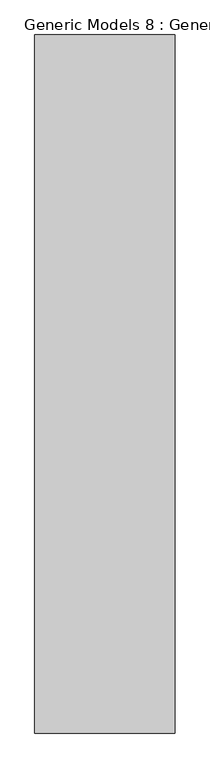
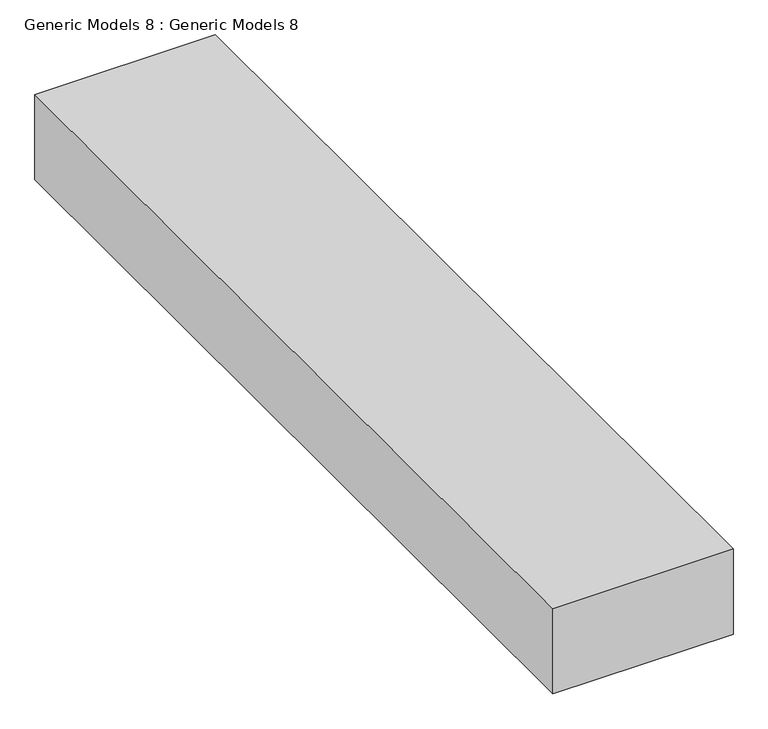
"""IFC4 building model written with IfcOpenShell, lengths in millimetres: proxy geometry, Generic Models 8 : Generic Models 8."""

from ifc_helpers import new_model, si_unit, frame, origin, place, context, project, spatial, polyline, outline, extrude, source, transform, mapped, element, save


def generic_models_8_generic_models_8_43166a7e(model_context):
    return source(origin(), model_context, "Body", "SweptSolid", [
        extrude(outline(polyline([(-14930.3656154, 3487.465781), (-14930.3656154, 5004.9260885), (-14625.5656154, 5004.9260885), (-14625.5656154, 3487.465781), (-14930.3656154, 3487.465781)])), frame((0.0, 0.0, 5181.6), z_axis=(0.0, 0.0, 1.0), x_axis=(1.0, 0.0, 0.0)), (0.0, 0.0, 1.0), 152.4),
    ])


if __name__ == "__main__":
    model = new_model("IFC4")
    model_context = context("Model", 3, world=origin())
    ifc_project = project(units=[si_unit("LENGTHUNIT", "METRE", prefix="MILLI")], contexts=[model_context])
    site = spatial("IfcSite", under=ifc_project)
    building = spatial("IfcBuilding", under=site)
    placement = place(None, origin())
    generic_models_8_generic_models_8_shape = generic_models_8_generic_models_8_43166a7e(model_context)
    element("IfcBuildingElementProxy", 1, Name="Generic Models 8 : Generic Models 8", ObjectType="Generic Models 8 : Generic Models 8", at=placement, inside=building, context=model_context, shape_type="MappedRepresentation", body=[
        mapped(generic_models_8_generic_models_8_shape, transform((0.0, 0.0, 0.0), x_axis=(1.0, 0.0, 0.0), y_axis=(0.0, 1.0, 0.0), z_axis=(0.0, 0.0, 1.0))),
    ])
    save(model, "model.ifc")

# Revit data of these elements
# Element 1 (IfcBuildingElementProxy, "Generic Models 8 : Generic Models 8")
#   Materials on its faces: "LIGHT BEIGE"
# Materials
#   "LIGHT BEIGE": class "Generic", colour RGB 120 120 120, transparency 0, Cost = 0
